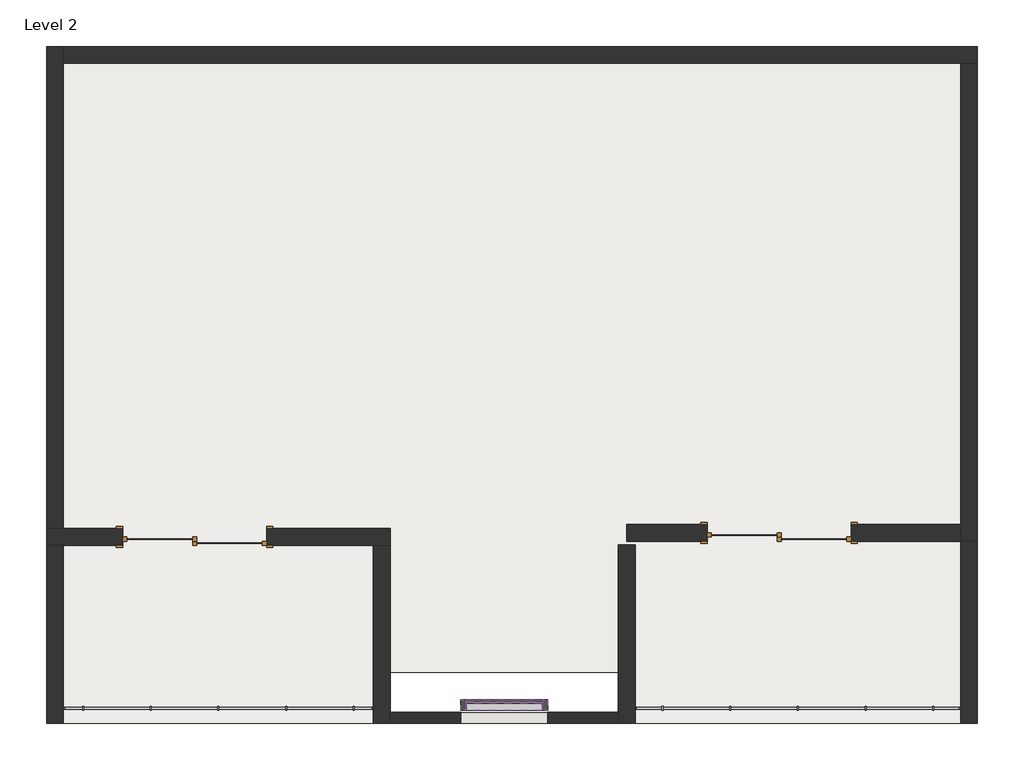
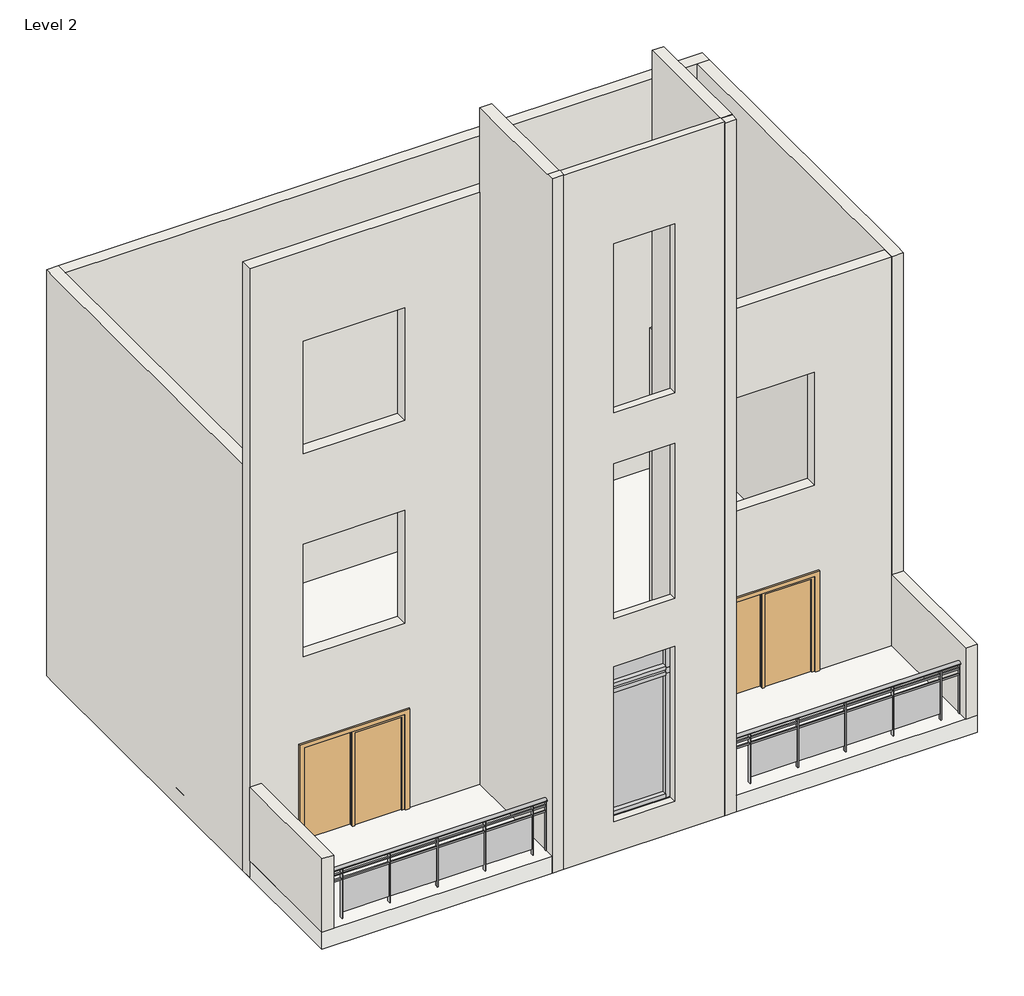
# One storey: 10 members, 10 walls, 3 plates, 2 doors, 2 railings, 1 roof.
"""IFC4 building model written with IfcOpenShell, lengths in millimetres."""

from ifc_helpers import new_model, si_unit, point, frame, origin, place, context, project, spatial, polyline, ellipse_curve, trimmed, outline, extrude, faceted_brep, transform, mapped, element, save
from ifc_brep_helpers import plane_surface, extruded_surface, advanced_brep
from components import door_076b30e0, member_d1708325, member_fb13da3b, member_15823cb3, member_73c23c35, member_410c6227, system_panel_glazed_14bb7e7b, system_panel_glazed_bdb1f896, system_panel_glazed_8073c085

model = new_model("IFC4")

# Units and contexts
model_context = context("Model", 3, world=origin())
ifc_project = project(units=[si_unit("LENGTHUNIT", "METRE", prefix="MILLI")], contexts=[model_context])

# Site, building, storey
site = spatial("IfcSite", under=ifc_project)
building = spatial("IfcBuilding", under=site)
storey = spatial("IfcBuildingStorey", under=building, Name="Level 2", Elevation=3657.6)

# Doors
placement = place(None, origin())
door_shape = door_076b30e0(model_context)
element("IfcDoor", 1, ObjectType="Door-Double-Sliding : 68\" x 80\"", at=placement, inside=storey, context=model_context, shape_type="MappedRepresentation", body=[
    mapped(door_shape, transform((-2221.0087885, 3717.6236997, 3657.6), x_axis=(-1.0, 0.0, 0.0), y_axis=(0.0, -1.0, 0.0), z_axis=(0.0, 0.0, 1.0))),
])
element("IfcDoor", 2, ObjectType="Door-Double-Sliding : 68\" x 80\"", at=placement, inside=storey, context=model_context, shape_type="MappedRepresentation", body=[
    mapped(door_shape, transform((-9238.1183714, 3666.8236997, 3657.6), x_axis=(-1.0, 0.0, 0.0), y_axis=(0.0, -1.0, 0.0), z_axis=(0.0, 0.0, 1.0))),
])

# Members
member_shape = member_d1708325(model_context)
element("IfcMember", 3, ObjectType="Rectangular Mullion : 2.5\" x 5\" rectangular", at=placement, inside=storey, context=model_context, shape_type="MappedRepresentation", body=[
    mapped(member_shape, transform((-6041.6537147, 1520.5236997, 6451.6), x_axis=(-1.0, 0.0, 0.0), y_axis=(0.0, -1.0, 0.0), z_axis=(0.0, 0.0, 1.0))),
])
member_2_shape = member_fb13da3b(model_context)
element("IfcMember", 4, ObjectType="Rectangular Mullion : 2.5\" x 5\" rectangular", at=placement, inside=storey, context=model_context, shape_type="MappedRepresentation", body=[
    mapped(member_2_shape, transform((-6041.6537147, 1520.5236997, 6553.2), x_axis=(-1.0, 0.0, 0.0), y_axis=(0.0, -1.0, 0.0), z_axis=(0.0, 0.0, 1.0))),
])
member_3_shape = member_15823cb3(model_context)
element("IfcMember", 5, ObjectType="Rectangular Mullion : 2.5\" x 5\" rectangular", at=placement, inside=storey, context=model_context, shape_type="MappedRepresentation", body=[
    mapped(member_3_shape, transform((-6041.6537147, 1520.5236997, 7010.4), x_axis=(-1.0, 0.0, 0.0), y_axis=(0.0, -1.0, 0.0), z_axis=(0.0, 0.0, 1.0))),
])
member_4_shape = member_73c23c35(model_context)
element("IfcMember", 6, ObjectType="Rectangular Mullion : 2.5\" x 5\" rectangular", at=placement, inside=storey, context=model_context, shape_type="MappedRepresentation", body=[
    mapped(member_4_shape, transform((-5978.1537147, 1520.5236997, 4216.4), x_axis=(0.0, 0.0, -1.0), y_axis=(0.0, -1.0, 0.0), z_axis=(-1.0, 0.0, 0.0))),
])
member_5_shape = member_410c6227(model_context)
element("IfcMember", 7, ObjectType="Rectangular Mullion : 2.5\" x 5\" rectangular", at=placement, inside=storey, context=model_context, shape_type="MappedRepresentation", body=[
    mapped(member_5_shape, transform((-5063.7537147, 1520.5236997, 6451.6), x_axis=(0.0, 0.0, 1.0), y_axis=(0.0, -1.0, 0.0), z_axis=(1.0, 0.0, 0.0))),
])
element("IfcMember", 8, ObjectType="Rectangular Mullion : 2.5\" x 5\" rectangular", at=placement, inside=storey, context=model_context, shape_type="MappedRepresentation", body=[
    mapped(member_5_shape, transform((-5063.7537147, 1520.5236997, 6553.2), x_axis=(0.0, 0.0, 1.0), y_axis=(0.0, -1.0, 0.0), z_axis=(1.0, 0.0, 0.0))),
])
element("IfcMember", 9, ObjectType="Rectangular Mullion : 2.5\" x 5\" rectangular", at=placement, inside=storey, context=model_context, shape_type="MappedRepresentation", body=[
    mapped(member_4_shape, transform((-5063.7537147, 1520.5236997, 7010.4), x_axis=(0.0, 0.0, 1.0), y_axis=(0.0, -1.0, 0.0), z_axis=(1.0, 0.0, 0.0))),
])
element("IfcMember", 10, ObjectType="Rectangular Mullion : 2.5\" x 5\" rectangular", at=placement, inside=storey, context=model_context, shape_type="MappedRepresentation", body=[
    mapped(member_2_shape, transform((-5000.2537147, 1520.5236997, 6451.6), x_axis=(1.0, 0.0, 0.0), y_axis=(0.0, -1.0, 0.0), z_axis=(0.0, 0.0, -1.0))),
])
element("IfcMember", 11, ObjectType="Rectangular Mullion : 2.5\" x 5\" rectangular", at=placement, inside=storey, context=model_context, shape_type="MappedRepresentation", body=[
    mapped(member_3_shape, transform((-5000.2537147, 1520.5236997, 6553.2), x_axis=(1.0, 0.0, 0.0), y_axis=(0.0, -1.0, 0.0), z_axis=(0.0, 0.0, -1.0))),
])
element("IfcMember", 12, ObjectType="Rectangular Mullion : 2.5\" x 5\" rectangular", at=placement, inside=storey, context=model_context, shape_type="MappedRepresentation", body=[
    mapped(member_shape, transform((-5000.2537147, 1520.5236997, 4216.4), x_axis=(1.0, 0.0, 0.0), y_axis=(0.0, -1.0, 0.0), z_axis=(0.0, 0.0, -1.0))),
])

# Plates
system_panel_glazed_shape = system_panel_glazed_14bb7e7b(model_context)
element("IfcPlate", 13, ObjectType="System Panel : Glazed", at=placement, inside=storey, context=model_context, shape_type="MappedRepresentation", body=[
    mapped(system_panel_glazed_shape, transform((-5520.9537147, 1520.5236997, 4279.9), x_axis=(1.0, 0.0, 0.0), y_axis=(0.0, 1.0, 0.0), z_axis=(0.0, 0.0, 1.0))),
])
system_panel_glazed_2_shape = system_panel_glazed_bdb1f896(model_context)
element("IfcPlate", 14, ObjectType="System Panel : Glazed", at=placement, inside=storey, context=model_context, shape_type="MappedRepresentation", body=[
    mapped(system_panel_glazed_2_shape, transform((-5520.9537147, 1520.5236997, 6584.95), x_axis=(1.0, 0.0, 0.0), y_axis=(0.0, 1.0, 0.0), z_axis=(0.0, 0.0, 1.0))),
])
system_panel_glazed_3_shape = system_panel_glazed_8073c085(model_context)
element("IfcPlate", 15, ObjectType="System Panel : Glazed", at=placement, inside=storey, context=model_context, shape_type="MappedRepresentation", body=[
    mapped(system_panel_glazed_3_shape, transform((-5520.9537147, 1520.5236997, 6483.35), x_axis=(1.0, 0.0, 0.0), y_axis=(0.0, 1.0, 0.0), z_axis=(0.0, 0.0, 1.0))),
])

# Railings
element("IfcRailing", 16, ObjectType="Glass Panel - Bottom Fill", at=placement, inside=storey, context=model_context, shape_type="SolidModel", body=[
    advanced_brep(
    [(-10812.9183714, 1520.5236997, 4876.8), (-10812.9183714, 1444.3236997, 4876.8), (-7091.896639, 1520.5236997, 4876.8), (-7091.896639, 1444.3236997, 4876.8)],
    [
        (0, 1, ellipse_curve(frame((-10812.9183714, 1482.4236997, 4876.8), z_axis=(-1.0, 0.0, 0.0), x_axis=(0.0, -1.0, 0.0)), 38.1, 28.575)),
        (1, 0, ellipse_curve(frame((-10812.9183714, 1482.4236997, 4876.8), z_axis=(-1.0, 0.0, 0.0), x_axis=(0.0, -1.0, 0.0)), 38.1, 28.575)),
        (2, 3, ellipse_curve(frame((-7091.896639, 1482.4236997, 4876.8), z_axis=(1.0, 0.0, 0.0), x_axis=(0.0, -1.0, 0.0)), 38.1, 28.575)),
        (3, 2, ellipse_curve(frame((-7091.896639, 1482.4236997, 4876.8), z_axis=(1.0, 0.0, 0.0), x_axis=(0.0, -1.0, 0.0)), 38.1, 28.575)),
        (0, 2),
        (3, 1),
    ],
    [
        plane_surface(frame((-10812.9183714, 1482.4236997, 4876.8), z_axis=(-1.0, 0.0, 0.0), x_axis=(0.0, 1.0, 0.0))),
        plane_surface(frame((-7091.896639, 1482.4236997, 4876.8), z_axis=(1.0, 0.0, 0.0), x_axis=(0.0, 1.0, 0.0))),
        extruded_surface(trimmed(ellipse_curve(frame((-7091.896639, 1482.4236997, 4876.8), z_axis=(-1.0, 0.0, 0.0), x_axis=(0.0, -1.0, 0.0)), 38.1, 28.575), [point((-7091.896639, 1520.5236997, 4876.8))], [point((-7091.896639, 1444.3236997, 4876.8))], True, "CARTESIAN"), (-3721.0217323999996, 0.0, 0.0), 3721.0217323999996),
        extruded_surface(trimmed(ellipse_curve(frame((-7091.896639, 1482.4236997, 4876.8), z_axis=(-1.0, 0.0, 0.0), x_axis=(0.0, -1.0, 0.0)), 38.1, 28.575), [point((-7091.896639, 1444.3236997, 4876.8))], [point((-7091.896639, 1520.5236997, 4876.8))], True, "CARTESIAN"), (-3721.0217323999996, 0.0, 0.0), 3721.0217323999996),
    ],
    [
        (0, [[1, 2]]),
        (1, [[3, 4]]),
        (2, [[-1, 5, -4, 6]]),
        (3, [[-2, -6, -3, -5]]),
    ],
),
    extrude(outline(polyline([(-10812.9183714, 1469.7236997), (-10812.9183714, 1495.1236997), (-7091.896639, 1495.1236997), (-7091.896639, 1469.7236997), (-10812.9183714, 1469.7236997)])), frame((0.0, 0.0, 4762.5), z_axis=(0.0, 0.0, 1.0), x_axis=(1.0, 0.0, 0.0)), (0.0, 0.0, 1.0), 25.4),
    extrude(outline(polyline([(-10812.9183714, 1469.7236997), (-10812.9183714, 1495.1236997), (-7091.896639, 1495.1236997), (-7091.896639, 1469.7236997), (-10812.9183714, 1469.7236997)])), frame((0.0, 0.0, 4660.9), z_axis=(0.0, 0.0, 1.0), x_axis=(1.0, 0.0, 0.0)), (0.0, 0.0, 1.0), 25.4),
    extrude(outline(polyline([(-7333.1575052, 1457.0236997), (-7333.1575052, 1507.8236997), (-7320.4575052, 1507.8236997), (-7320.4575052, 1457.0236997), (-7333.1575052, 1457.0236997)])), frame((0.0, 0.0, 3962.4), z_axis=(0.0, 0.0, 1.0), x_axis=(1.0, 0.0, 0.0)), (0.0, 0.0, 1.0), 885.6788223),
    extrude(outline(polyline([(-8139.6075052, 1488.9588567), (-7326.8075052, 1488.9588567), (-7326.8075052, 1482.6088567), (-8139.6075052, 1482.6088567), (-8139.6075052, 1488.9588567)])), frame((0.0, 0.0, 4064.0), z_axis=(0.0, 0.0, 1.0), x_axis=(1.0, 0.0, 0.0)), (0.0, 0.0, 1.0), 596.9),
    extrude(outline(polyline([(-8145.9575052, 1457.0236997), (-8145.9575052, 1507.8236997), (-8133.2575052, 1507.8236997), (-8133.2575052, 1457.0236997), (-8145.9575052, 1457.0236997)])), frame((0.0, 0.0, 3962.4), z_axis=(0.0, 0.0, 1.0), x_axis=(1.0, 0.0, 0.0)), (0.0, 0.0, 1.0), 885.6788223),
    extrude(outline(polyline([(-8952.4075052, 1488.9588567), (-8139.6075052, 1488.9588567), (-8139.6075052, 1482.6088567), (-8952.4075052, 1482.6088567), (-8952.4075052, 1488.9588567)])), frame((0.0, 0.0, 4064.0), z_axis=(0.0, 0.0, 1.0), x_axis=(1.0, 0.0, 0.0)), (0.0, 0.0, 1.0), 596.9),
    extrude(outline(polyline([(-8958.7575052, 1457.0236997), (-8958.7575052, 1507.8236997), (-8946.0575052, 1507.8236997), (-8946.0575052, 1457.0236997), (-8958.7575052, 1457.0236997)])), frame((0.0, 0.0, 3962.4), z_axis=(0.0, 0.0, 1.0), x_axis=(1.0, 0.0, 0.0)), (0.0, 0.0, 1.0), 885.6788223),
    extrude(outline(polyline([(-9765.2075052, 1488.9588567), (-8952.4075052, 1488.9588567), (-8952.4075052, 1482.6088567), (-9765.2075052, 1482.6088567), (-9765.2075052, 1488.9588567)])), frame((0.0, 0.0, 4064.0), z_axis=(0.0, 0.0, 1.0), x_axis=(1.0, 0.0, 0.0)), (0.0, 0.0, 1.0), 596.9),
    extrude(outline(polyline([(-9771.5575052, 1457.0236997), (-9771.5575052, 1507.8236997), (-9758.8575052, 1507.8236997), (-9758.8575052, 1457.0236997), (-9771.5575052, 1457.0236997)])), frame((0.0, 0.0, 3962.4), z_axis=(0.0, 0.0, 1.0), x_axis=(1.0, 0.0, 0.0)), (0.0, 0.0, 1.0), 885.6788223),
    extrude(outline(polyline([(-10578.0075052, 1488.9588567), (-9765.2075052, 1488.9588567), (-9765.2075052, 1482.6088567), (-10578.0075052, 1482.6088567), (-10578.0075052, 1488.9588567)])), frame((0.0, 0.0, 4064.0), z_axis=(0.0, 0.0, 1.0), x_axis=(1.0, 0.0, 0.0)), (0.0, 0.0, 1.0), 596.9),
    extrude(outline(polyline([(-10584.3575052, 1457.0236997), (-10584.3575052, 1507.8236997), (-10571.6575052, 1507.8236997), (-10571.6575052, 1457.0236997), (-10584.3575052, 1457.0236997)])), frame((0.0, 0.0, 3962.4), z_axis=(0.0, 0.0, 1.0), x_axis=(1.0, 0.0, 0.0)), (0.0, 0.0, 1.0), 885.6788223),
    extrude(outline(polyline([(-7104.596639, 1472.8986997), (-7104.596639, 1491.9486997), (-7085.546639, 1491.9486997), (-7085.546639, 1472.8986997), (-7104.596639, 1472.8986997)])), frame((0.0, 0.0, 3962.4), z_axis=(0.0, 0.0, 1.0), x_axis=(1.0, 0.0, 0.0)), (0.0, 0.0, 1.0), 885.6788223),
    extrude(outline(polyline([(-10819.2683714, 1472.8986997), (-10819.2683714, 1491.9486997), (-10800.2183714, 1491.9486997), (-10800.2183714, 1472.8986997), (-10819.2683714, 1472.8986997)])), frame((0.0, 0.0, 3962.4), z_axis=(0.0, 0.0, 1.0), x_axis=(1.0, 0.0, 0.0)), (0.0, 0.0, 1.0), 885.6788223),
])
element("IfcRailing", 17, ObjectType="Glass Panel - Bottom Fill", at=placement, inside=storey, context=model_context, shape_type="SolidModel", body=[
    advanced_brep(
    [(-3948.2087885, 1520.5236997, 4876.8), (-3948.2087885, 1444.3236997, 4876.8), (-43.3183714, 1520.5236997, 4876.8), (-43.3183714, 1444.3236997, 4876.8)],
    [
        (0, 1, ellipse_curve(frame((-3948.2087885, 1482.4236997, 4876.8), z_axis=(-1.0, 0.0, 0.0), x_axis=(0.0, -1.0, 0.0)), 38.1, 28.575)),
        (1, 0, ellipse_curve(frame((-3948.2087885, 1482.4236997, 4876.8), z_axis=(-1.0, 0.0, 0.0), x_axis=(0.0, -1.0, 0.0)), 38.1, 28.575)),
        (2, 3, ellipse_curve(frame((-43.3183714, 1482.4236997, 4876.8), z_axis=(1.0, 0.0, 0.0), x_axis=(0.0, -1.0, 0.0)), 38.1, 28.575)),
        (3, 2, ellipse_curve(frame((-43.3183714, 1482.4236997, 4876.8), z_axis=(1.0, 0.0, 0.0), x_axis=(0.0, -1.0, 0.0)), 38.1, 28.575)),
        (0, 2),
        (3, 1),
    ],
    [
        plane_surface(frame((-3948.2087885, 1482.4236997, 4876.8), z_axis=(-1.0, 0.0, 0.0), x_axis=(0.0, 1.0, 0.0))),
        plane_surface(frame((-43.3183714, 1482.4236997, 4876.8), z_axis=(1.0, 0.0, 0.0), x_axis=(0.0, 1.0, 0.0))),
        extruded_surface(trimmed(ellipse_curve(frame((-43.3183714, 1482.4236997, 4876.8), z_axis=(-1.0, 0.0, 0.0), x_axis=(0.0, -1.0, 0.0)), 38.1, 28.575), [point((-43.3183714, 1520.5236997, 4876.8))], [point((-43.3183714, 1444.3236997, 4876.8))], True, "CARTESIAN"), (-3904.8904171, 0.0, 0.0), 3904.8904171),
        extruded_surface(trimmed(ellipse_curve(frame((-43.3183714, 1482.4236997, 4876.8), z_axis=(-1.0, 0.0, 0.0), x_axis=(0.0, -1.0, 0.0)), 38.1, 28.575), [point((-43.3183714, 1444.3236997, 4876.8))], [point((-43.3183714, 1520.5236997, 4876.8))], True, "CARTESIAN"), (-3904.8904171, 0.0, 0.0), 3904.8904171),
    ],
    [
        (0, [[1, 2]]),
        (1, [[3, 4]]),
        (2, [[-1, 5, -4, 6]]),
        (3, [[-2, -6, -3, -5]]),
    ],
),
    extrude(outline(polyline([(-3948.2087885, 1469.7236997), (-3948.2087885, 1495.1236997), (-43.3183714, 1495.1236997), (-43.3183714, 1469.7236997), (-3948.2087885, 1469.7236997)])), frame((0.0, 0.0, 4762.5), z_axis=(0.0, 0.0, 1.0), x_axis=(1.0, 0.0, 0.0)), (0.0, 0.0, 1.0), 25.4),
    extrude(outline(polyline([(-3948.2087885, 1469.7236997), (-3948.2087885, 1495.1236997), (-43.3183714, 1495.1236997), (-43.3183714, 1469.7236997), (-3948.2087885, 1469.7236997)])), frame((0.0, 0.0, 4660.9), z_axis=(0.0, 0.0, 1.0), x_axis=(1.0, 0.0, 0.0)), (0.0, 0.0, 1.0), 25.4),
    extrude(outline(polyline([(-376.51358, 1457.0236997), (-376.51358, 1507.8236997), (-363.81358, 1507.8236997), (-363.81358, 1457.0236997), (-376.51358, 1457.0236997)])), frame((0.0, 0.0, 3962.4), z_axis=(0.0, 0.0, 1.0), x_axis=(1.0, 0.0, 0.0)), (0.0, 0.0, 1.0), 885.6788223),
    extrude(outline(polyline([(-1182.96358, 1488.9588567), (-370.16358, 1488.9588567), (-370.16358, 1482.6088567), (-1182.96358, 1482.6088567), (-1182.96358, 1488.9588567)])), frame((0.0, 0.0, 4064.0), z_axis=(0.0, 0.0, 1.0), x_axis=(1.0, 0.0, 0.0)), (0.0, 0.0, 1.0), 596.9),
    extrude(outline(polyline([(-1189.31358, 1457.0236997), (-1189.31358, 1507.8236997), (-1176.61358, 1507.8236997), (-1176.61358, 1457.0236997), (-1189.31358, 1457.0236997)])), frame((0.0, 0.0, 3962.4), z_axis=(0.0, 0.0, 1.0), x_axis=(1.0, 0.0, 0.0)), (0.0, 0.0, 1.0), 885.6788223),
    extrude(outline(polyline([(-1995.76358, 1488.9588567), (-1182.96358, 1488.9588567), (-1182.96358, 1482.6088567), (-1995.76358, 1482.6088567), (-1995.76358, 1488.9588567)])), frame((0.0, 0.0, 4064.0), z_axis=(0.0, 0.0, 1.0), x_axis=(1.0, 0.0, 0.0)), (0.0, 0.0, 1.0), 596.9),
    extrude(outline(polyline([(-2002.11358, 1457.0236997), (-2002.11358, 1507.8236997), (-1989.41358, 1507.8236997), (-1989.41358, 1457.0236997), (-2002.11358, 1457.0236997)])), frame((0.0, 0.0, 3962.4), z_axis=(0.0, 0.0, 1.0), x_axis=(1.0, 0.0, 0.0)), (0.0, 0.0, 1.0), 885.6788223),
    extrude(outline(polyline([(-2808.56358, 1488.9588567), (-1995.76358, 1488.9588567), (-1995.76358, 1482.6088567), (-2808.56358, 1482.6088567), (-2808.56358, 1488.9588567)])), frame((0.0, 0.0, 4064.0), z_axis=(0.0, 0.0, 1.0), x_axis=(1.0, 0.0, 0.0)), (0.0, 0.0, 1.0), 596.9),
    extrude(outline(polyline([(-2814.91358, 1457.0236997), (-2814.91358, 1507.8236997), (-2802.21358, 1507.8236997), (-2802.21358, 1457.0236997), (-2814.91358, 1457.0236997)])), frame((0.0, 0.0, 3962.4), z_axis=(0.0, 0.0, 1.0), x_axis=(1.0, 0.0, 0.0)), (0.0, 0.0, 1.0), 885.6788223),
    extrude(outline(polyline([(-3621.36358, 1488.9588567), (-2808.56358, 1488.9588567), (-2808.56358, 1482.6088567), (-3621.36358, 1482.6088567), (-3621.36358, 1488.9588567)])), frame((0.0, 0.0, 4064.0), z_axis=(0.0, 0.0, 1.0), x_axis=(1.0, 0.0, 0.0)), (0.0, 0.0, 1.0), 596.9),
    extrude(outline(polyline([(-3627.71358, 1457.0236997), (-3627.71358, 1507.8236997), (-3615.01358, 1507.8236997), (-3615.01358, 1457.0236997), (-3627.71358, 1457.0236997)])), frame((0.0, 0.0, 3962.4), z_axis=(0.0, 0.0, 1.0), x_axis=(1.0, 0.0, 0.0)), (0.0, 0.0, 1.0), 885.6788223),
    extrude(outline(polyline([(-56.0183714, 1472.8986997), (-56.0183714, 1491.9486997), (-36.9683714, 1491.9486997), (-36.9683714, 1472.8986997), (-56.0183714, 1472.8986997)])), frame((0.0, 0.0, 3962.4), z_axis=(0.0, 0.0, 1.0), x_axis=(1.0, 0.0, 0.0)), (0.0, 0.0, 1.0), 885.6788223),
    extrude(outline(polyline([(-3954.5587885, 1472.8986997), (-3954.5587885, 1491.9486997), (-3935.5087885, 1491.9486997), (-3935.5087885, 1472.8986997), (-3954.5587885, 1472.8986997)])), frame((0.0, 0.0, 3962.4), z_axis=(0.0, 0.0, 1.0), x_axis=(1.0, 0.0, 0.0)), (0.0, 0.0, 1.0), 885.6788223),
])

# Roof
element("IfcRoof", 18, ObjectType="Generic - 12\"", at=placement, inside=storey, context=model_context, shape_type="SweptSolid", body=[
    extrude(outline(polyline([(-11016.1183714, 9432.6236997), (159.8816286, 9432.6236997), (159.8816286, 1304.6236997), (-3948.2087885, 1304.6236997), (-3948.2087885, 1914.2236997), (-7091.896639, 1914.2236997), (-7091.896639, 1304.6236997), (-11016.1183714, 1304.6236997), (-11016.1183714, 9432.6236997)])), frame((0.0, 0.0, 3657.6), z_axis=(0.0, 0.0, 1.0), x_axis=(1.0, 0.0, 0.0)), (0.0, 0.0, 1.0), 304.8),
])

# Walls
element("IfcWall", 19, ObjectType="Generic - 5\"", at=placement, inside=storey, context=model_context, shape_type="Brep", body=[
    faceted_brep([(-6888.696639, 1304.6236997, 3657.6), (-4151.4087885, 1304.6236997, 3657.6), (-4151.4087885, 1304.6236997, 16144.9059158), (-4151.4087885, 1304.6236997, 16163.7107538), (-6888.696639, 1304.6236997, 16163.7107538), (-5000.2537147, 1304.6236997, 14630.4), (-5000.2537147, 1304.6236997, 11582.4), (-6041.6537147, 1304.6236997, 11582.4), (-6041.6537147, 1304.6236997, 14630.4), (-5000.2537147, 1304.6236997, 10668.0), (-5000.2537147, 1304.6236997, 7874.0), (-6041.6537147, 1304.6236997, 7874.0), (-6041.6537147, 1304.6236997, 10668.0), (-5000.2537147, 1304.6236997, 7010.4), (-5000.2537147, 1304.6236997, 4216.4), (-6041.6537147, 1304.6236997, 4216.4), (-6041.6537147, 1304.6236997, 7010.4), (-6888.696639, 1431.6236997, 3657.6), (-6888.696639, 1431.6236997, 16154.4), (-6888.696639, 1431.6236997, 16163.7107538), (-4151.4087885, 1431.6236997, 16163.7107538), (-4151.4087885, 1431.6236997, 3657.6), (-5000.2537147, 1431.6236997, 14630.4), (-6041.6537147, 1431.6236997, 14630.4), (-6041.6537147, 1431.6236997, 11582.4), (-5000.2537147, 1431.6236997, 11582.4), (-5000.2537147, 1431.6236997, 10668.0), (-6041.6537147, 1431.6236997, 10668.0), (-6041.6537147, 1431.6236997, 7874.0), (-5000.2537147, 1431.6236997, 7874.0), (-5000.2537147, 1431.6236997, 7010.4), (-6041.6537147, 1431.6236997, 7010.4), (-6041.6537147, 1431.6236997, 4216.4), (-5000.2537147, 1431.6236997, 4216.4)], [[[0, 1, 2, 3, 4], [5, 6, 7, 8], [9, 10, 11, 12], [13, 14, 15, 16]], [[17, 18, 19, 20, 21], [22, 23, 24, 25], [26, 27, 28, 29], [30, 31, 32, 33]], [[1, 0, 17, 21]], [[4, 3, 20, 19]], [[6, 5, 22, 25]], [[7, 6, 25, 24]], [[8, 7, 24, 23]], [[5, 8, 23, 22]], [[10, 9, 26, 29]], [[11, 10, 29, 28]], [[12, 11, 28, 27]], [[9, 12, 27, 26]], [[14, 13, 30, 33]], [[15, 14, 33, 32]], [[16, 15, 32, 31]], [[13, 16, 31, 30]], [[0, 4, 19, 18, 17]], [[3, 2, 1, 21, 20]]]),
])
element("IfcWall", 20, ObjectType="Generic - 8\"", at=placement, inside=storey, context=model_context, shape_type="Brep", body=[
    faceted_brep([(-11016.1183714, 3438.2236997, 3657.6), (-10101.7183714, 3438.2236997, 3657.6), (-10101.7183714, 3438.2236997, 5689.6), (-8374.5183714, 3438.2236997, 5689.6), (-8374.5183714, 3438.2236997, 3657.6), (-7091.896639, 3438.2236997, 3657.6), (-6888.696639, 3438.2236997, 3657.6), (-6888.696639, 3438.2236997, 14630.4), (-11016.1183714, 3438.2236997, 14630.4), (-11016.1183714, 3438.2236997, 10972.8), (-11016.1183714, 3438.2236997, 7315.2), (-11016.1183714, 3438.2236997, 5285.2547339), (-11016.1183714, 3438.2236997, 3962.4), (-8374.5183714, 3438.2236997, 9347.2), (-8374.5183714, 3438.2236997, 7315.2), (-10101.7183714, 3438.2236997, 7315.2), (-10101.7183714, 3438.2236997, 9347.2), (-8374.5183714, 3438.2236997, 13004.8), (-8374.5183714, 3438.2236997, 10972.8), (-10101.7183714, 3438.2236997, 10972.8), (-10101.7183714, 3438.2236997, 13004.8), (-10101.7183714, 3641.4236997, 5689.6), (-10101.7183714, 3641.4236997, 3657.6), (-10812.9183714, 3641.4236997, 3657.6), (-11016.1183714, 3641.4236997, 3657.6), (-11016.1183714, 3641.4236997, 7315.2), (-11016.1183714, 3641.4236997, 10972.8), (-11016.1183714, 3641.4236997, 14630.4), (-10812.9183714, 3641.4236997, 14630.4), (-6888.696639, 3641.4236997, 14630.4), (-6888.696639, 3641.4236997, 3657.6), (-8374.5183714, 3641.4236997, 3657.6), (-8374.5183714, 3641.4236997, 5689.6), (-8374.5183714, 3641.4236997, 9347.2), (-10101.7183714, 3641.4236997, 9347.2), (-10101.7183714, 3641.4236997, 7315.2), (-8374.5183714, 3641.4236997, 7315.2), (-8374.5183714, 3641.4236997, 13004.8), (-10101.7183714, 3641.4236997, 13004.8), (-10101.7183714, 3641.4236997, 10972.8), (-8374.5183714, 3641.4236997, 10972.8)], [[[0, 1, 2, 3, 4, 5, 6, 7, 8, 9, 10, 11, 12], [13, 14, 15, 16], [17, 18, 19, 20]], [[21, 22, 23, 24, 25, 26, 27, 28, 29, 30, 31, 32], [33, 34, 35, 36], [37, 38, 39, 40]], [[31, 30, 6, 5, 4]], [[24, 23, 22, 1, 0]], [[8, 7, 29, 28, 27]], [[7, 6, 30, 29]], [[4, 3, 32, 31]], [[2, 1, 22, 21]], [[3, 2, 21, 32]], [[14, 13, 33, 36]], [[15, 14, 36, 35]], [[16, 15, 35, 34]], [[13, 16, 34, 33]], [[18, 17, 37, 40]], [[19, 18, 40, 39]], [[20, 19, 39, 38]], [[17, 20, 38, 37]], [[8, 27, 26, 25, 24, 0, 12, 11, 10, 9]]]),
])
element("IfcWall", 21, ObjectType="Generic - 8\"", at=placement, inside=storey, context=model_context, shape_type="Brep", body=[
    faceted_brep([(-10812.9183714, 3641.4236997, 10972.8), (-10812.9183714, 3641.4236997, 3657.6), (-10812.9183714, 9229.4236997, 3657.6), (-10812.9183714, 9432.6236997, 3657.6), (-10812.9183714, 9432.6236997, 7315.2), (-10812.9183714, 9432.6236997, 10972.8), (-10812.9183714, 9229.4236997, 10972.8), (-11016.1183714, 3641.4236997, 3657.6), (-11016.1183714, 3641.4236997, 10972.8), (-11016.1183714, 9229.4236997, 10972.8), (-11016.1183714, 9432.6236997, 10972.8), (-11016.1183714, 9432.6236997, 3657.6), (-11016.1183714, 9229.4236997, 3657.6)], [[[0, 1, 2, 3, 4, 5, 6]], [[7, 8, 9, 10, 11, 12]], [[3, 2, 1, 7, 12, 11]], [[0, 6, 5, 10, 9, 8]], [[0, 8, 7, 1]], [[3, 11, 10, 5, 4]]]),
])
element("IfcWall", 22, ObjectType="Generic - 8\"", at=placement, inside=storey, context=model_context, shape_type="Brep", body=[
    faceted_brep([(-10812.9183714, 9229.4236997, 10972.8), (-10812.9183714, 9229.4236997, 3657.6), (-43.3183714, 9229.4236997, 3657.6), (159.8816286, 9229.4236997, 3657.6), (159.8816286, 9229.4236997, 7315.2), (159.8816286, 9229.4236997, 10972.8), (-43.3183714, 9229.4236997, 10972.8), (-10812.9183714, 9432.6236997, 3657.6), (-10812.9183714, 9432.6236997, 10972.8), (-43.3183714, 9432.6236997, 10972.8), (159.8816286, 9432.6236997, 10972.8), (159.8816286, 9432.6236997, 3657.6), (-43.3183714, 9432.6236997, 3657.6)], [[[0, 1, 2, 3, 4, 5, 6]], [[7, 8, 9, 10, 11, 12]], [[3, 2, 1, 7, 12, 11]], [[0, 6, 5, 10, 9, 8]], [[3, 11, 10, 5, 4]], [[0, 8, 7, 1]]]),
])
element("IfcWall", 23, ObjectType="Generic - 8\"", at=placement, inside=storey, context=model_context, shape_type="Brep", body=[
    faceted_brep([(-43.3183714, 9229.4236997, 10972.8), (-43.3183714, 9229.4236997, 3657.6), (-43.3183714, 3692.2236997, 3657.6), (-43.3183714, 3489.0236997, 3657.6), (-43.3183714, 3489.0236997, 3962.4), (-43.3183714, 3489.0236997, 5239.7319996), (-43.3183714, 3489.0236997, 7315.2), (-43.3183714, 3489.0236997, 10972.8), (-43.3183714, 3692.2236997, 10972.8), (159.8816286, 9229.4236997, 3657.6), (159.8816286, 9229.4236997, 10972.8), (159.8816286, 3692.2236997, 10972.8), (159.8816286, 3489.0236997, 10972.8), (159.8816286, 3489.0236997, 7315.2), (159.8816286, 3489.0236997, 5239.7319996), (159.8816286, 3489.0236997, 3962.4), (159.8816286, 3489.0236997, 3657.6)], [[[0, 1, 2, 3, 4, 5, 6, 7, 8]], [[9, 10, 11, 12, 13, 14, 15, 16]], [[3, 2, 1, 9, 16]], [[0, 8, 7, 12, 11, 10]], [[3, 16, 15, 14, 13, 12, 7, 6, 5, 4]], [[0, 10, 9, 1]]]),
])
element("IfcWall", 24, ObjectType="Generic - 8\"", at=placement, inside=storey, context=model_context, shape_type="Brep", body=[
    faceted_brep([(-3084.6087885, 3692.2236997, 5689.6), (-3084.6087885, 3692.2236997, 3657.6), (-4049.8087885, 3692.2236997, 3657.6), (-4049.8087885, 3692.2236997, 10972.8), (-43.3183714, 3692.2236997, 10972.8), (-43.3183714, 3692.2236997, 3657.6), (-1357.4087885, 3692.2236997, 3657.6), (-1357.4087885, 3692.2236997, 5689.6), (-1357.4087885, 3692.2236997, 9347.2), (-3084.6087885, 3692.2236997, 9347.2), (-3084.6087885, 3692.2236997, 7315.2), (-1408.2087885, 3692.2236997, 7315.2), (-1357.4087885, 3692.2236997, 7315.2), (-4049.8087885, 3489.0236997, 3657.6), (-3084.6087885, 3489.0236997, 3657.6), (-3084.6087885, 3489.0236997, 5689.6), (-1357.4087885, 3489.0236997, 5689.6), (-1357.4087885, 3489.0236997, 3657.6), (-43.3183714, 3489.0236997, 3657.6), (-43.3183714, 3489.0236997, 10972.8), (-4049.8087885, 3489.0236997, 10972.8), (-1357.4087885, 3489.0236997, 9347.2), (-1357.4087885, 3489.0236997, 7315.2), (-1408.2087885, 3489.0236997, 7315.2), (-3084.6087885, 3489.0236997, 7315.2), (-3084.6087885, 3489.0236997, 9347.2)], [[[0, 1, 2, 3, 4, 5, 6, 7], [8, 9, 10, 11, 12]], [[13, 14, 15, 16, 17, 18, 19, 20], [21, 22, 23, 24, 25]], [[6, 5, 18, 17]], [[2, 1, 14, 13]], [[3, 2, 13, 20]], [[4, 3, 20, 19]], [[22, 21, 8, 12]], [[24, 23, 22, 12, 11, 10]], [[25, 24, 10, 9]], [[21, 25, 9, 8]], [[17, 16, 7, 6]], [[15, 14, 1, 0]], [[16, 15, 0, 7]], [[4, 19, 18, 5]]]),
])
element("IfcWall", 25, ObjectType="Generic - 8\"", at=placement, inside=storey, context=model_context, shape_type="Brep", body=[
    faceted_brep([(-4151.4087885, 3444.5736997, 3657.6), (-4151.4087885, 1431.6236997, 3657.6), (-4151.4087885, 1304.6236997, 3657.6), (-4151.4087885, 1304.6236997, 16144.9059158), (-4151.4087885, 1431.6236997, 16144.9059158), (-4151.4087885, 1431.6236997, 16154.4), (-4151.4087885, 3444.5736997, 16154.4), (-3948.2087885, 3444.5736997, 3657.6), (-3948.2087885, 3444.5736997, 16154.4), (-3948.2087885, 1431.6236997, 16154.4), (-3948.2087885, 1431.6236997, 16144.9059158), (-3948.2087885, 1304.6236997, 16144.9059158), (-3948.2087885, 1304.6236997, 3657.6)], [[[0, 1, 2, 3, 4, 5, 6]], [[7, 8, 9, 10, 11, 12]], [[2, 1, 0, 7, 12]], [[0, 6, 8, 7]], [[4, 3, 11, 10]], [[4, 10, 9, 5]], [[6, 5, 9, 8]], [[3, 2, 12, 11]]]),
])
element("IfcWall", 26, ObjectType="Generic - 8\"", at=placement, inside=storey, context=model_context, shape_type="Brep", body=[
    faceted_brep([(-7091.896639, 3438.2236997, 3657.6), (-7091.896639, 1304.6236997, 3657.6), (-7091.896639, 1304.6236997, 16172.9844909), (-7091.896639, 1431.6236997, 16172.9844909), (-7091.896639, 1431.6236997, 16154.4), (-7091.896639, 3438.2236997, 16154.4), (-6888.696639, 3438.2236997, 3657.6), (-6888.696639, 3438.2236997, 14630.4), (-6888.696639, 3438.2236997, 16154.4), (-6888.696639, 1431.6236997, 16154.4), (-6888.696639, 1431.6236997, 16163.7107538), (-6888.696639, 1431.6236997, 16172.9844909), (-6888.696639, 1304.6236997, 16172.9844909), (-6888.696639, 1304.6236997, 16163.7107538), (-6888.696639, 1304.6236997, 3657.6), (-6888.696639, 1431.6236997, 3657.6)], [[[0, 1, 2, 3, 4, 5]], [[6, 7, 8, 9, 10, 11, 12, 13, 14, 15]], [[1, 0, 6, 15, 14]], [[0, 5, 8, 7, 6]], [[3, 2, 12, 11]], [[3, 11, 10, 9, 4]], [[5, 4, 9, 8]], [[2, 1, 14, 13, 12]]]),
])
element("IfcWall", 27, ObjectType="Generic - 8\"", at=placement, inside=storey, context=model_context, shape_type="SweptSolid", body=[
    extrude(outline(polyline([(-11016.1183714, 1304.6236997), (-11016.1183714, 3438.2236997), (-10812.9183714, 3438.2236997), (-10812.9183714, 1304.6236997), (-11016.1183714, 1304.6236997)])), frame((0.0, 0.0, 3962.4), z_axis=(0.0, 0.0, 1.0), x_axis=(1.0, 0.0, 0.0)), (0.0, 0.0, 1.0), 1322.8547339),
])
element("IfcWall", 28, ObjectType="Generic - 8\"", at=placement, inside=storey, context=model_context, shape_type="SweptSolid", body=[
    extrude(outline(polyline([(-43.3183714, 1304.6236997), (-43.3183714, 3489.0236997), (159.8816286, 3489.0236997), (159.8816286, 1304.6236997), (-43.3183714, 1304.6236997)])), frame((0.0, 0.0, 3962.4), z_axis=(0.0, 0.0, 1.0), x_axis=(1.0, 0.0, 0.0)), (0.0, 0.0, 1.0), 1277.3319996),
])

save(model, "model.ifc")

# Revit data of these elements
# Type "Door-Double-Sliding : 68\" x 80\""
#   Type Mark = "11"
#   Construction Type Id = "opn-d45"
#   Assembly Code = "C1020"
#   Analytic Construction = "Wood frame, double glass door "
#   Thickness = 0' - 2"
#   Thermal Resistance (R) = 1.8150 (h·ft²·°F)/BTU
#   Heat Transfer Coefficient (U) = 0.5510 BTU/(h·ft²·°F)
#   Height = 6' - 8"
#   Rail Width = 0' - 2"
#   Stiles = 0' - 2"
#   Trim Projection Ext = 0' - 1"
#   Trim Projection Int = 0' - 1"
#   Trim Width = 0' - 3"
#   Width = 5' - 8"
#   Define Thermal Properties by = 1
#   Glazing = Glass
#   Panel Material = Wood - Birch - Solid Stained Light Low Gloss
#   Trim Material = Paint - Sienna
#   Visual Light Transmittance = 0
#   Solar Heat Gain Coefficient = 0
#   Function = (empty or 0)
#   Wall Closure = (empty or 0)
# Type "Rectangular Mullion : 2.5\" x 5\" rectangular"
#   built-in parameter 1007304 = 0.416667 (stored number, unit not read)
#   built-in parameter 1007301 = 0.104167 (stored number, unit not read)
#   built-in parameter 1007300 = 0.104167 (stored number, unit not read)
# Type "System Panel : Glazed"
#   Construction Type Id = "GSP4R"
#   Analytic Construction = "1/8 in Pilkington single glazing"
#   Visual Light Transmittance = 0.9
#   Solar Heat Gain Coefficient = 0.86
#   Heat Transfer Coefficient (U) = 1.18115 BTU/(h·ft²·°F)
# Type "Glass Panel - Bottom Fill"
#   Assembly Code = "C2010400"
#   built-in parameter 1008612 = 0.0416667 (stored number, unit not read)
#   built-in parameter 1008611 = 0.0416667 (stored number, unit not read)
#   built-in parameter 1008609 = 0.333333 (stored number, unit not read)
#   built-in parameter 1008604 = 0.166667 (stored number, unit not read)
#   built-in parameter 1008603 = 0.166667 (stored number, unit not read)
#   Railing Height = 3' - 0"
#   built-in parameter 1008630 = 2
#   built-in parameter 1008610 = 2
#   built-in parameter 1008618 = Baluster - Square : 3/4"
# Type "Generic - 12\""
#   Assembly Code = "B1020"
#   Layers, outside or top first: 1' - 0" no material (function 1)
# Type "Generic - 5\""
#   Assembly Code = "B2010"
#   Layers, outside or top first: 0' - 5" no material (function 1)
# Type "Generic - 8\""
#   Assembly Code = "B2010"
#   Layers, outside or top first: 0' - 8" no material (function 1)
# Elements 1, 2 (IfcDoor, "Door-Double-Sliding : 68\" x 80\"")
#   Phase Created = New Construction
#   Materials on its faces: "Paint - Sienna", "Wood - Birch - Solid Stained Light Low Gloss", "Glass"
# Elements 3, 4, 5, 6, 7, 8, 9, 10, 11, 12 (IfcMember, "Rectangular Mullion : 2.5\" x 5\" rectangular")
#   Phase Created = New Construction
#   Materials on its faces: "Aluminum"
# Elements 13, 14, 15 (IfcPlate, "System Panel : Glazed")
#   Phase Created = New Construction
#   Materials on its faces: "Glass"
# Elements 16, 17 (IfcRailing, "Glass Panel - Bottom Fill")
#   built-in parameter 1008621 = 1 (stored number, unit not read)
#   Phase Created = New Construction
#   Materials on its faces: "Glass"
# Element 18 (IfcRoof, "Generic - 12\"")
#   built-in parameter 1001705 = 13 (stored number, unit not read)
#   built-in parameter 1001710 = 33615
#   Phase Created = New Construction
#   Materials on its faces: "Default Roof"
# Element 19 (IfcWall, "Generic - 5\"")
#   Top Offset = 29' - 0.36657"
#   Base Offset = 0' - 0"
#   wall height = 41' - 0.36657"
#   Phase Created = New Construction
#   Base Constraint = Level 2
#   Top Constraint = Level 3
#   Materials on its faces: "Default Wall"
# Element 20 (IfcWall, "Generic - 8\"")
#   Top Offset = 24' - 0"
#   Base Offset = 0' - 0"
#   wall height = 36' - 0"
#   Phase Created = New Construction
#   Base Constraint = Level 2
#   Top Constraint = Level 3
#   Materials on its faces: "Default Wall"
# Elements 21, 22, 23, 24 (IfcWall, "Generic - 8\"")
#   Top Offset = 0' - 0"
#   Base Offset = 0' - 0"
#   Unconnected Height = 24' - 0"
#   wall height = 24' - 0"
#   Phase Created = New Construction
#   Base Constraint = Level 2
#   Materials on its faces: "Default Wall"
# Element 25 (IfcWall, "Generic - 8\"")
#   Top Offset = 0' - 0"
#   Base Offset = 0' - 0"
#   Unconnected Height = 40' - 11.62622"
#   wall height = 40' - 11.62622"
#   Phase Created = New Construction
#   Base Constraint = Level 2
#   Materials on its faces: "Default Wall"
# Element 26 (IfcWall, "Generic - 8\"")
#   Top Offset = 0' - 0"
#   Base Offset = 0' - 0"
#   Unconnected Height = 41' - 0.73167"
#   wall height = 41' - 0.73167"
#   Phase Created = New Construction
#   Base Constraint = Level 2
#   Materials on its faces: "Default Wall"
# Element 27 (IfcWall, "Generic - 8\"")
#   built-in parameter 1001111 = 1' - 0"
#   Top Offset = 0' - 0"
#   Base Offset = 1' - 0"
#   Unconnected Height = 4' - 4.0809"
#   wall height = 4' - 4.0809"
#   Phase Created = New Construction
#   Base Constraint = Level 2
#   Materials on its faces: "Default Wall"
# Element 28 (IfcWall, "Generic - 8\"")
#   built-in parameter 1001111 = 1' - 0"
#   Top Offset = 0' - 0"
#   Base Offset = 1' - 0"
#   Unconnected Height = 4' - 2.28866"
#   wall height = 4' - 2.28866"
#   Phase Created = New Construction
#   Base Constraint = Level 2
#   Materials on its faces: "Default Wall"
# Materials
#   "Glass": class "Glass", colour RGB 0 128 192, transparency 0.75, Description = "Soda Lime Glass", Cost = 0
#   "Wood - Birch - Solid Stained Light Low Gloss": class "Wood", colour RGB 210 159 95, transparency 0, Cost = 0
#   "Paint - Sienna": colour RGB 118 70 51, transparency 0, Cost = 0
#   "Aluminum": class "Metal", colour RGB 247 247 247, transparency 0, Description = "Aluminum 6061", Cost = 0
#   "Default Roof": colour RGB 88 101 114, transparency 0
#   "Default Wall": colour RGB 128 128 128, transparency 0
